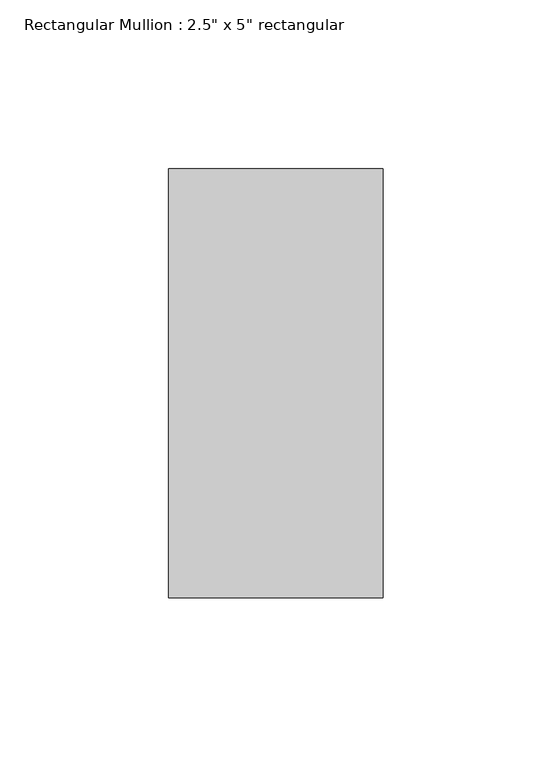
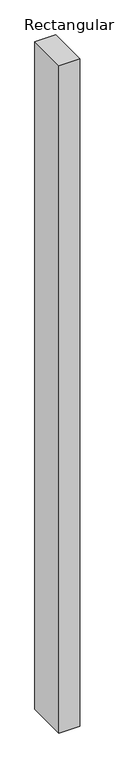
"""IFC4 building model written with IfcOpenShell, lengths in millimetres: member geometry."""

from ifc_helpers import new_model, si_unit, frame, origin, place, context, project, spatial, polyline, outline, extrude, source, transform, mapped, element, save


def member_fb65e0d5(model_context):
    return source(origin(), model_context, "Body", "SweptSolid", [
        extrude(outline(polyline([(31.75, 63.5), (31.75, -63.5), (-31.75, -63.5), (-31.75, 63.5), (31.75, 63.5)])), frame((0.0, 0.0, -2159.0), z_axis=(0.0, 0.0, 1.0), x_axis=(1.0, 0.0, 0.0)), (0.0, 0.0, 1.0), 2159.0),
    ])


if __name__ == "__main__":
    model = new_model("IFC4")
    model_context = context("Model", 3, world=origin())
    ifc_project = project(units=[si_unit("LENGTHUNIT", "METRE", prefix="MILLI")], contexts=[model_context])
    site = spatial("IfcSite", under=ifc_project)
    building = spatial("IfcBuilding", under=site)
    placement = place(None, origin())
    member_shape = member_fb65e0d5(model_context)
    element("IfcMember", 1, ObjectType="Rectangular Mullion : 2.5\" x 5\" rectangular", at=placement, inside=building, context=model_context, shape_type="MappedRepresentation", body=[
        mapped(member_shape, transform((0.0, 0.0, 0.0), x_axis=(1.0, 0.0, 0.0), y_axis=(0.0, 1.0, 0.0), z_axis=(0.0, 0.0, 1.0))),
    ])
    save(model, "model.ifc")

# Revit data of these elements
# Type "Rectangular Mullion : 2.5\" x 5\" rectangular"
#   built-in parameter 1007304 = 0.416667 (stored number, unit not read)
#   built-in parameter 1007301 = 0.104167 (stored number, unit not read)
#   built-in parameter 1007300 = 0.104167 (stored number, unit not read)
